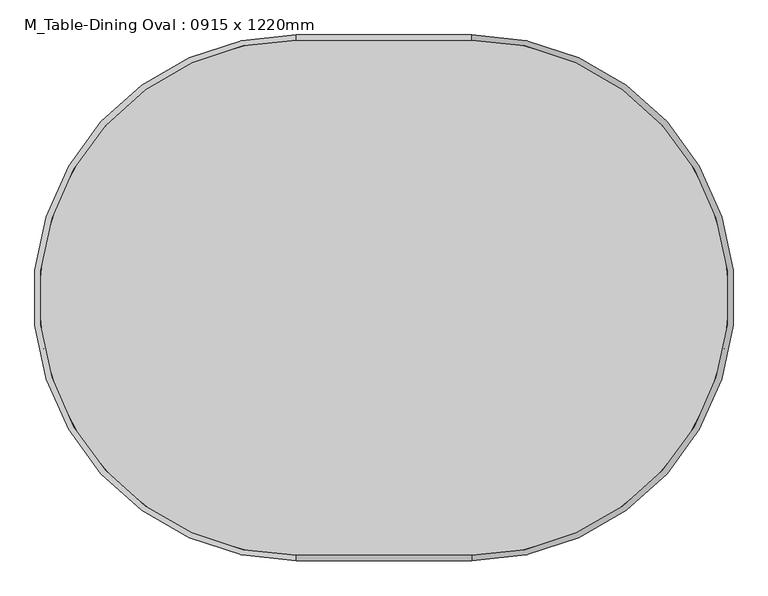
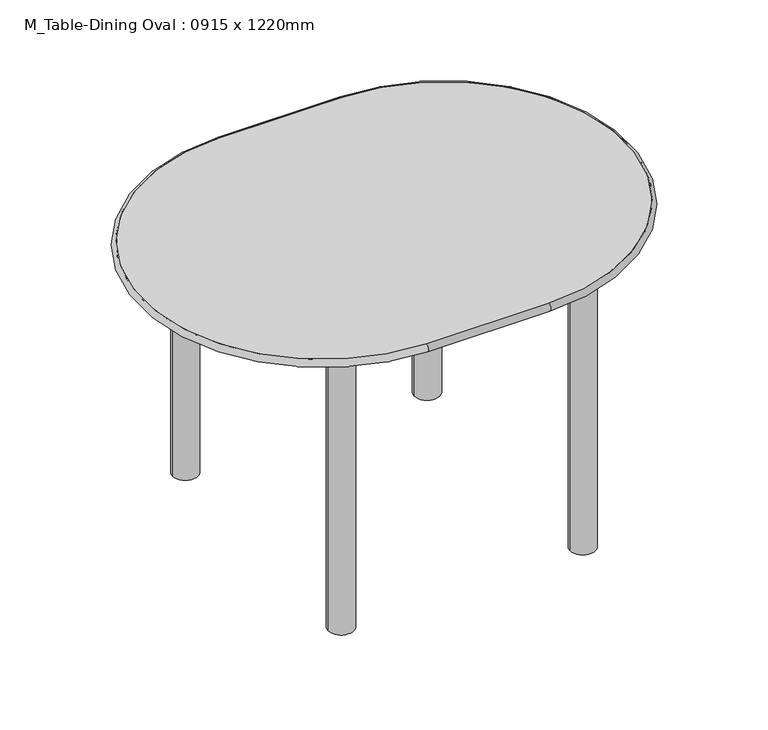
"""IFC4 building model written with IfcOpenShell, lengths in millimetres: furniture geometry, M_Table-Dining Oval : 0915 x 1220mm."""

from ifc_helpers import new_model, si_unit, point, frame, frame_2d, origin, origin_with_axes, place, context, project, spatial, polyline, circle_curve, ellipse_curve, trimmed, segment, composite_curve, outline, extrude, source, transform, mapped, element, save
from ifc_brep_helpers import plane_surface, cylinder_surface, revolved_surface, advanced_brep


def m_table_dining_oval_0915_x_1220mm_c3de6a6b(model_context):
    return source(origin(), model_context, "Body", "SolidModel", [
        advanced_brep(
        [(-554.3196721, -806.0733607, 762.0), (-554.3196721, -806.0733607, 742.95), (-249.3196721, -806.0733607, 742.95), (-249.3196721, -806.0733607, 762.0), (-249.3196721, 89.8766393, 762.0), (-249.3196721, 89.8766393, 742.95), (-554.3196721, 89.8766393, 742.95), (-554.3196721, 89.8766393, 762.0)],
        [
            (0, 1, circle_curve(frame((-554.3196721, -806.0733607, 752.475), z_axis=(1.0, 0.0, 0.0), x_axis=(0.0, 1.0, 0.0)), 9.525)),
            (1, 2),
            (2, 3, circle_curve(frame((-249.3196721, -806.0733607, 752.475), z_axis=(-1.0, 0.0, 0.0), x_axis=(0.0, 1.0, 0.0)), 9.525)),
            (3, 0),
            (1, 0),
            (3, 2),
            (4, 3, circle_curve(frame((-249.3196721, -358.0983607, 762.0), z_axis=(0.0, 0.0, -1.0), x_axis=(0.0, -1.0, 0.0)), 447.975)),
            (2, 5, circle_curve(frame((-249.3196721, -358.0983607, 742.95), z_axis=(0.0, 0.0, 1.0), x_axis=(0.0, -1.0, 0.0)), 447.975)),
            (5, 4, circle_curve(frame((-249.3196721, 89.8766393, 752.475), z_axis=(1.0, 0.0, 0.0), x_axis=(0.0, -1.0, 0.0)), 9.525)),
            (4, 5),
            (5, 6),
            (6, 7, circle_curve(frame((-554.3196721, 89.8766393, 752.475), z_axis=(1.0, 0.0, 0.0), x_axis=(0.0, -1.0, 0.0)), 9.525)),
            (7, 4),
            (7, 6),
            (0, 7, circle_curve(frame((-554.3196721, -358.0983607, 762.0), z_axis=(0.0, 0.0, -1.0), x_axis=(0.0, 1.0, 0.0)), 447.975)),
            (6, 1, circle_curve(frame((-554.3196721, -358.0983607, 742.95), z_axis=(0.0, 0.0, 1.0), x_axis=(0.0, 1.0, 0.0)), 447.975)),
        ],
        [
            cylinder_surface(frame((-554.3196721, -806.0733607, 752.475), z_axis=(-1.0, 0.0, 0.0), x_axis=(0.0, 1.0, 0.0)), 9.525),
            plane_surface(frame((-554.3196721, -806.0733607, 762.0), z_axis=(0.0, 1.0, 0.0), x_axis=(1.0, 0.0, 0.0))),
            revolved_surface(trimmed(ellipse_curve(frame((-249.3196721, -806.0733607, 752.475), z_axis=(-1.0, 0.0, 0.0), x_axis=(0.0, 1.0, 0.0)), 9.525, 9.525), [point((-249.3196721, -806.0733607, 742.95))], [point((-249.3196721, -806.0733607, 762.0))], True, "CARTESIAN"), (-249.3196721, -358.0983607, 0.0), (0.0, 0.0, 1.0)),
            revolved_surface(polyline([(-249.3196721, -806.0733607, 762.0), (-249.3196721, -806.0733607, 742.95)]), (-249.3196721, -358.0983607, 0.0), (0.0, 0.0, 1.0)),
            cylinder_surface(frame((-249.3196721, 89.8766393, 752.475), z_axis=(1.0, 0.0, 0.0), x_axis=(0.0, -1.0, 0.0)), 9.525),
            plane_surface(frame((-249.3196721, 89.8766393, 762.0), z_axis=(0.0, -1.0, 0.0), x_axis=(-1.0, 0.0, 0.0))),
            revolved_surface(trimmed(ellipse_curve(frame((-554.3196721, 89.8766393, 752.475), z_axis=(1.0, 0.0, 0.0), x_axis=(0.0, -1.0, 0.0)), 9.525, 9.525), [point((-554.3196721, 89.8766393, 742.95))], [point((-554.3196721, 89.8766393, 762.0))], True, "CARTESIAN"), (-554.3196721, -358.0983607, 0.0), (0.0, 0.0, 1.0)),
            revolved_surface(polyline([(-554.3196721, 89.87663930000002, 762.0), (-554.3196721, 89.87663930000002, 742.95)]), (-554.3196721, -358.0983607, 0.0), (0.0, 0.0, 1.0)),
        ],
        [
            (0, [[1, 2, 3, 4]]),
            (1, [[5, -4, 6, -2]]),
            (2, [[7, -3, 8, 9]]),
            (3, [[-8, -6, -7, 10]]),
            (4, [[-9, 11, 12, 13]]),
            (5, [[-10, -13, 14, -11]]),
            (6, [[15, -12, 16, -1]]),
            (7, [[-16, -14, -15, -5]]),
        ],
    ),
        extrude(outline(composite_curve([segment(trimmed(circle_curve(frame_2d((-703.5446721, -21.2483607)), 31.75), [point((-735.2946721, -21.2483607))], [point((-671.7946721, -21.2483607))], False, "CARTESIAN"), True, "CONTINUOUS"), segment(trimmed(circle_curve(frame_2d((-703.5446721, -21.2483607)), 31.75), [point((-671.7946721, -21.2483607))], [point((-735.2946721, -21.2483607))], False, "CARTESIAN"), True, "CONTINUOUS")], self_intersect=False)), origin_with_axes(), (0.0, 0.0, 1.0), 742.95),
        extrude(outline(composite_curve([segment(trimmed(circle_curve(frame_2d((-703.5446721, -694.9483607)), 31.75), [point((-735.2946721, -694.9483607))], [point((-671.7946721, -694.9483607))], False, "CARTESIAN"), True, "CONTINUOUS"), segment(trimmed(circle_curve(frame_2d((-703.5446721, -694.9483607)), 31.75), [point((-671.7946721, -694.9483607))], [point((-735.2946721, -694.9483607))], False, "CARTESIAN"), True, "CONTINUOUS")], self_intersect=False)), origin_with_axes(), (0.0, 0.0, 1.0), 742.95),
        extrude(outline(composite_curve([segment(trimmed(circle_curve(frame_2d((-100.0946721, -21.2483607)), 31.75), [point((-131.8446721, -21.2483607))], [point((-68.3446721, -21.2483607))], False, "CARTESIAN"), True, "CONTINUOUS"), segment(trimmed(circle_curve(frame_2d((-100.0946721, -21.2483607)), 31.75), [point((-68.3446721, -21.2483607))], [point((-131.8446721, -21.2483607))], False, "CARTESIAN"), True, "CONTINUOUS")], self_intersect=False)), origin_with_axes(), (0.0, 0.0, 1.0), 742.95),
        extrude(outline(composite_curve([segment(trimmed(circle_curve(frame_2d((-100.0946721, -694.9483607)), 31.75), [point((-131.8446721, -694.9483607))], [point((-68.3446721, -694.9483607))], False, "CARTESIAN"), True, "CONTINUOUS"), segment(trimmed(circle_curve(frame_2d((-100.0946721, -694.9483607)), 31.75), [point((-68.3446721, -694.9483607))], [point((-131.8446721, -694.9483607))], False, "CARTESIAN"), True, "CONTINUOUS")], self_intersect=False)), origin_with_axes(), (0.0, 0.0, 1.0), 742.95),
        extrude(outline(polyline([(-81.0446721, -2.1983607), (-81.0446721, -713.9983607), (-722.5946721, -713.9983607), (-722.5946721, -2.1983607), (-81.0446721, -2.1983607)]), holes=[polyline([(-100.0946721, -21.2483607), (-703.5446721, -21.2483607), (-703.5446721, -694.9483607), (-100.0946721, -694.9483607), (-100.0946721, -21.2483607)])]), frame((0.0, 0.0, 692.15), z_axis=(0.0, 0.0, 1.0), x_axis=(1.0, 0.0, 0.0)), (0.0, 0.0, 1.0), 50.8),
        extrude(outline(composite_curve([segment(polyline([(-554.3196721, 89.8766393), (-249.3196721, 89.8766393)]), True, "CONTINUOUS"), segment(trimmed(circle_curve(frame_2d((-249.3196721, -358.0983607)), 447.975), [point((-249.3196721, 89.8766393))], [point((198.6553279, -358.0983607))], False, "CARTESIAN"), True, "CONTINUOUS"), segment(trimmed(circle_curve(frame_2d((-249.3196721, -358.0983607)), 447.975), [point((198.6553279, -358.0983607))], [point((-249.3196721, -806.0733607))], False, "CARTESIAN"), True, "CONTINUOUS"), segment(polyline([(-249.3196721, -806.0733607), (-554.3196721, -806.0733607)]), True, "CONTINUOUS"), segment(trimmed(circle_curve(frame_2d((-554.3196721, -358.0983607)), 447.975), [point((-554.3196721, -806.0733607))], [point((-1002.2946721, -358.0983607))], False, "CARTESIAN"), True, "CONTINUOUS"), segment(trimmed(circle_curve(frame_2d((-554.3196721, -358.0983607)), 447.975), [point((-1002.2946721, -358.0983607))], [point((-554.3196721, 89.8766393))], False, "CARTESIAN"), True, "CONTINUOUS")], self_intersect=False)), frame((0.0, 0.0, 742.95), z_axis=(0.0, 0.0, 1.0), x_axis=(1.0, 0.0, 0.0)), (0.0, 0.0, 1.0), 19.05),
    ])


if __name__ == "__main__":
    model = new_model("IFC4")
    model_context = context("Model", 3, world=origin())
    ifc_project = project(units=[si_unit("LENGTHUNIT", "METRE", prefix="MILLI")], contexts=[model_context])
    site = spatial("IfcSite", under=ifc_project)
    building = spatial("IfcBuilding", under=site)
    placement = place(None, origin())
    m_table_dining_oval_0915_x_1220mm_shape = m_table_dining_oval_0915_x_1220mm_c3de6a6b(model_context)
    element("IfcFurniture", 1, ObjectType="M_Table-Dining Oval : 0915 x 1220mm", at=placement, inside=building, context=model_context, shape_type="MappedRepresentation", body=[
        mapped(m_table_dining_oval_0915_x_1220mm_shape, transform((0.0, 0.0, 0.0), x_axis=(1.0, 0.0, 0.0), y_axis=(0.0, 1.0, 0.0), z_axis=(0.0, 0.0, 1.0))),
    ])
    save(model, "model.ifc")

# Revit data of these elements
# Type "M_Table-Dining Oval : 0915 x 1220mm"
#   Length = 4' - 0.0315"
#   Width = 3' - 0.02362"
#   Base Material = none
#   Top Material = none
#   Default Elevation = 0
# Element 1 (IfcFurniture, "M_Table-Dining Oval : 0915 x 1220mm")
#   Materials on its faces: "Glass - Clear, Grey"
# Materials
#   "Glass - Clear, Grey": class "Glass", colour RGB 252 255 255, transparency 0.64
